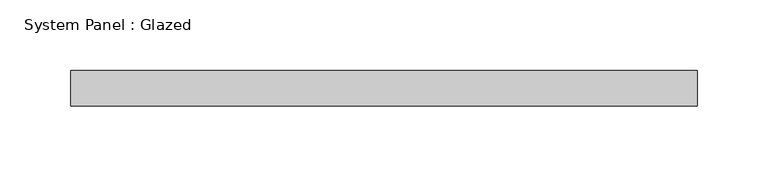
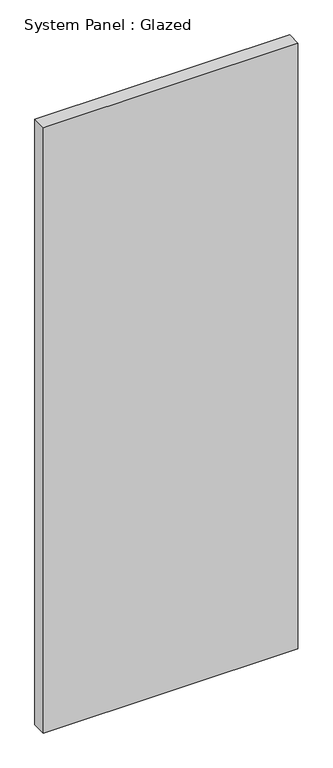
"""IFC4 building model written with IfcOpenShell, lengths in millimetres: plate geometry, System Panel : Glazed."""

from ifc_helpers import new_model, si_unit, origin, origin_with_axes, place, context, project, spatial, polyline, outline, extrude, source, transform, mapped, element, save


def system_panel_glazed_a23f7966(model_context):
    return source(origin(), model_context, "Body", "SweptSolid", [
        extrude(outline(polyline([(222.25, 19.05), (-222.25, 19.05), (-222.25, 44.45), (222.25, 44.45), (222.25, 19.05)])), origin_with_axes(), (0.0, 0.0, 1.0), 1117.6),
    ])


if __name__ == "__main__":
    model = new_model("IFC4")
    model_context = context("Model", 3, world=origin())
    ifc_project = project(units=[si_unit("LENGTHUNIT", "METRE", prefix="MILLI")], contexts=[model_context])
    site = spatial("IfcSite", under=ifc_project)
    building = spatial("IfcBuilding", under=site)
    placement = place(None, origin())
    system_panel_glazed_shape = system_panel_glazed_a23f7966(model_context)
    element("IfcPlate", 1, ObjectType="System Panel : Glazed", at=placement, inside=building, context=model_context, shape_type="MappedRepresentation", body=[
        mapped(system_panel_glazed_shape, transform((0.0, 0.0, 0.0), x_axis=(1.0, 0.0, 0.0), y_axis=(0.0, 1.0, 0.0), z_axis=(0.0, 0.0, 1.0))),
    ])
    save(model, "model.ifc")

# Revit data of these elements
# Type "System Panel : Glazed"
#   Construction Type Id = "GSP4R"
#   Analytic Construction = "1/8 in Pilkington single glazing"
#   Visual Light Transmittance = 0.9
#   Solar Heat Gain Coefficient = 0.86
#   Heat Transfer Coefficient (U) = 1.18115 BTU/(h·ft²·°F)
#   Define Thermal Properties by = 1
# Element 1 (IfcPlate, "System Panel : Glazed")
#   Materials on its faces: "Glass"
# Materials
#   "Glass": class "Glass", colour RGB 0 128 192, transparency 0.75, Description = "Soda Lime Glass", Cost = 0
